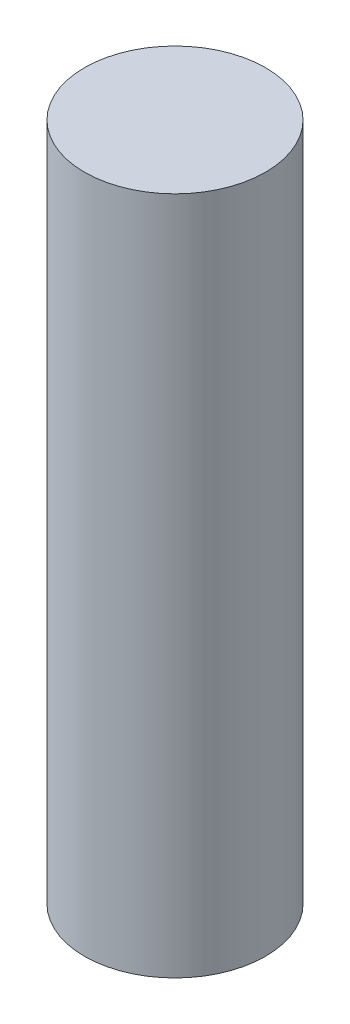
from build123d import *

# Parameters (mm, degrees)
SHANK_PROFILE_12_R = 6
SHANK_12X45_DEPTH  = 22.5


with BuildPart() as part:
    # Shank Profile Ø12 → Shank Ø12x45 (new, symmetric)
    with BuildSketch(Plane(origin=(0, 0, 0), x_dir=(1, 0, 0), z_dir=(0, 1, 0))):
        with Locations(Location((0, 0, 0), (0, 0, 90))):
            Circle(SHANK_PROFILE_12_R)
    extrude(amount=SHANK_12X45_DEPTH, both=True)


solid = part.part
